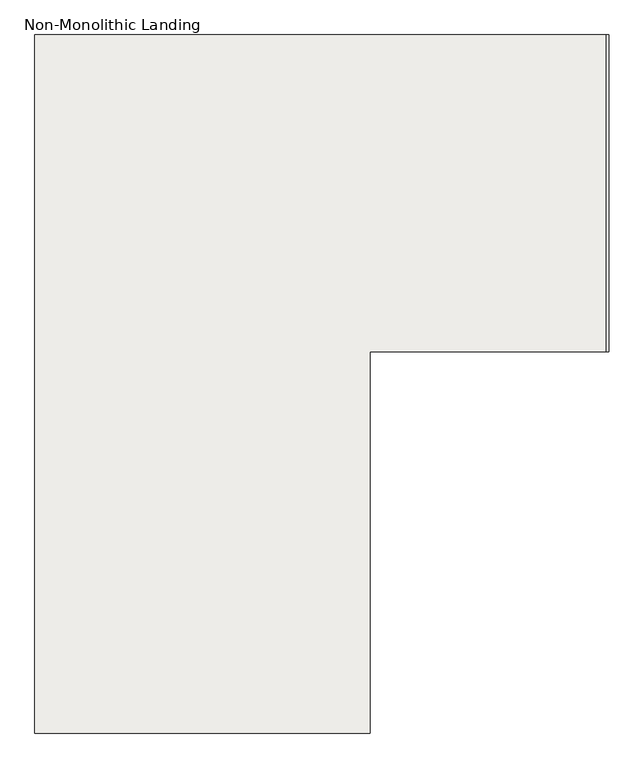
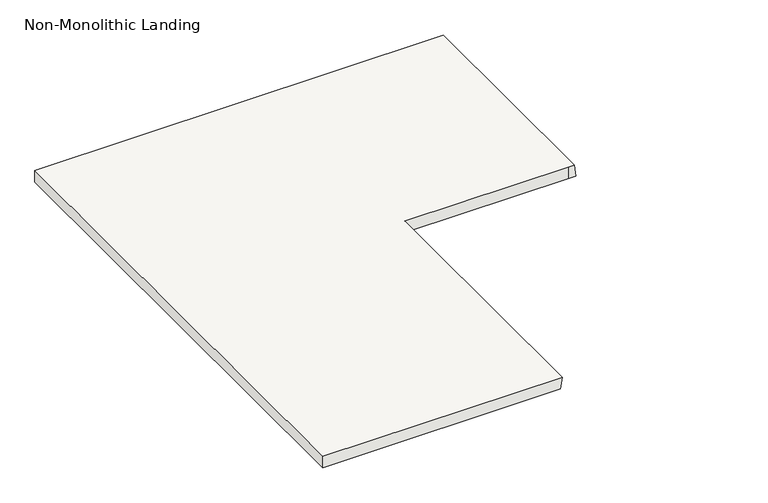
"""IFC4 building model written with IfcOpenShell, lengths in millimetres: slab geometry, Non-Monolithic Landing."""

from ifc_helpers import new_model, si_unit, origin, place, context, project, spatial, faceted_brep, source, transform, mapped, element, save


def non_monolithic_landing_e0a5ec0f(model_context):
    return source(origin(), model_context, "Body", "Brep", [
        faceted_brep([(-1207.4697153, 1980.9593033, 1043.4782609), (-1200.2822153, 1980.9593033, 993.4782609), (-1200.2822153, 2926.2309464, 993.4782609), (-1207.4697153, 2926.2309464, 1043.4782609), (-1914.0915237, 1810.8567276, 1043.4782609), (-1914.0915237, 1980.9593033, 1043.4782609), (-1232.4697153, 1980.9593033, 1043.4782609), (-1232.4697153, 2926.2309464, 1043.4782609), (-2914.117305, 2926.2309464, 1043.4782609), (-2914.117305, 843.0180557, 1043.4782609), (-1914.0915237, 843.0180557, 1043.4782609), (-1914.0915237, 1980.9593033, 993.4782609), (-1914.0915237, 1810.8567276, 993.4782609), (-1921.2790237, 1810.8567276, 993.4782609), (-1921.2790237, 843.0180557, 993.4782609), (-2914.117305, 843.0180557, 993.4782609), (-2914.117305, 2926.2309464, 993.4782609), (-1232.4697153, 2926.2309464, 993.4782609), (-1232.4697153, 1980.9593033, 993.4782609)], [[[0, 1, 2, 3]], [[4, 5, 6, 0, 3, 7, 8, 9, 10]], [[11, 12, 13, 14, 15, 16, 17, 2, 1, 18]], [[5, 4, 12, 11]], [[6, 5, 11, 18]], [[0, 6, 18, 1]], [[7, 3, 2, 17]], [[8, 7, 17, 16]], [[9, 8, 16, 15]], [[10, 9, 15, 14]], [[4, 13, 12]], [[13, 4, 10, 14]]]),
    ])


if __name__ == "__main__":
    model = new_model("IFC4")
    model_context = context("Model", 3, world=origin())
    ifc_project = project(units=[si_unit("LENGTHUNIT", "METRE", prefix="MILLI")], contexts=[model_context])
    site = spatial("IfcSite", under=ifc_project)
    building = spatial("IfcBuilding", under=site)
    placement = place(None, origin())
    non_monolithic_landing_shape = non_monolithic_landing_e0a5ec0f(model_context)
    element("IfcSlab", 1, ObjectType="Non-Monolithic Landing", at=placement, inside=building, context=model_context, shape_type="MappedRepresentation", body=[
        mapped(non_monolithic_landing_shape, transform((0.0, 0.0, 0.0), x_axis=(1.0, 0.0, 0.0), y_axis=(0.0, 1.0, 0.0), z_axis=(0.0, 0.0, 1.0))),
    ])
    save(model, "model.ifc")
